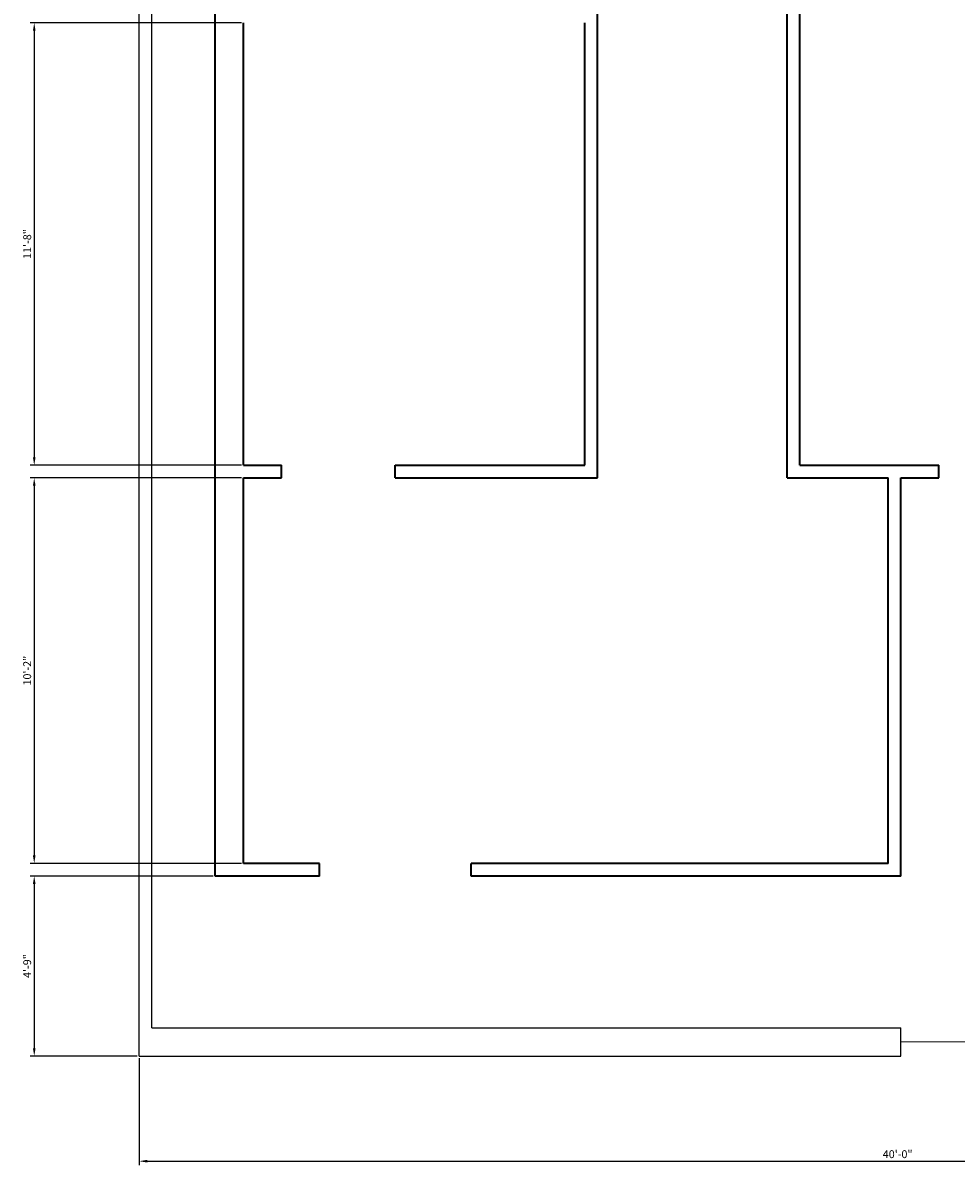
# Model space of a CAD drawing. Units: inches. Extents: x 2169 to 10664, y 1669 to 6352.
# Tile 9 of 17: x 4397 to 4692, y 1968 to 2329. Entities that reach past the tile are written whole.
import ezdxf

# ---------------------------------------------------------------- set-up
doc = ezdxf.new("R2010")
doc.units = ezdxf.units.IN
for name, color, linetype, lineweight in [('A-ANNO-DIMS', 3, 'Continuous', 18), ('A-DOOR', 4, 'Continuous', 18), ('A-WALL', 7, 'Continuous', 35), ('C-PROP', 251, 'Continuous', 25)]:
    doc.layers.add(name, color=color, linetype=linetype, lineweight=lineweight)
doc.styles.get("Standard").update_dxf_attribs({"font": 'arial.ttf'})
doc.dimstyles.new('ISO-25', dxfattribs={"dimtxt": 2.5, "dimasz": 2.5, "dimexe": 1.25, "dimexo": 0.625, "dimtad": 1, "dimdec": 0, "dimlunit": 3, "dimtxsty": 'Standard', "dimcen": 2.5, "dimadec": 0, "dimazin": 0, "dimtfac": 1, "dimtdec": 0, "dimtmove": 0, "dimatfit": 3, "dimfxl": 1, "dimarcsym": 0})

# ---------------------------------------------------------------- blocks, each defined once
blk = doc.blocks.new('*D102')
at = {"layer": 'A-ANNO-DIMS', "color": 0, "lineweight": -2, "transparency": 16777216}
for p, q in [((4433.57, 2001.56), (4433.57, 1967.69)), ((4913.57, 2001.56), (4913.57, 1967.69)), ((4436.07, 1968.94), (4911.07, 1968.94))]:
    blk.add_line(p, q, dxfattribs=at)
at = {"layer": 'A-ANNO-DIMS', "color": 0, "transparency": 16777216}
for points in [[(4436.07, 1969.36), (4436.07, 1968.52), (4433.57, 1968.94)], [(4911.07, 1969.36), (4911.07, 1968.52), (4913.57, 1968.94)]]:
    blk.add_solid(points, dxfattribs=at)
at = {"layer": 'Defpoints', "color": 0, "transparency": 16777216}
for p in [(4433.57, 2002.19), (4913.57, 2002.19), (4913.57, 1968.94)]:
    blk.add_point(p, dxfattribs=at)
at = {"layer": 'A-ANNO-DIMS', "color": 0, "transparency": 16777216, "insert": (4673.57, 1970.84), "char_height": 2.5, "attachment_point": 5}
blk.add_mtext('40\'-0"', dxfattribs=at)
blk = doc.blocks.new('*D114')
at = {"layer": 'A-ANNO-DIMS', "color": 0, "lineweight": -2, "transparency": 16777216}
for p, q in [((4465.95, 2329.19), (4399.07, 2329.19)), ((4400.32, 2326.69), (4400.32, 2191.69)), ((4465.95, 2189.19), (4399.07, 2189.19))]:
    blk.add_line(p, q, dxfattribs=at)
at = {"layer": 'A-ANNO-DIMS', "color": 0, "transparency": 16777216}
for points in [[(4399.91, 2326.69), (4400.74, 2326.69), (4400.32, 2329.19)], [(4399.91, 2191.69), (4400.74, 2191.69), (4400.32, 2189.19)]]:
    blk.add_solid(points, dxfattribs=at)
at = {"layer": 'Defpoints', "color": 0, "transparency": 16777216}
for p in [(4466.57, 2329.19), (4400.32, 2189.19), (4466.57, 2189.19)]:
    blk.add_point(p, dxfattribs=at)
at = {"layer": 'A-ANNO-DIMS', "color": 0, "transparency": 16777216, "insert": (4398.42, 2259.19), "char_height": 2.5, "attachment_point": 5, "rotation": 90}
blk.add_mtext('11\'-8"', dxfattribs=at)
blk = doc.blocks.new('*D115')
at = {"layer": 'A-ANNO-DIMS', "color": 0, "lineweight": -2, "transparency": 16777216}
for p, q in [((4465.95, 2185.19), (4399.07, 2185.19)), ((4400.32, 2182.69), (4400.32, 2065.69)), ((4465.95, 2063.19), (4399.07, 2063.19))]:
    blk.add_line(p, q, dxfattribs=at)
at = {"layer": 'A-ANNO-DIMS', "color": 0, "transparency": 16777216}
for points in [[(4399.91, 2182.69), (4400.74, 2182.69), (4400.32, 2185.19)], [(4399.91, 2065.69), (4400.74, 2065.69), (4400.32, 2063.19)]]:
    blk.add_solid(points, dxfattribs=at)
at = {"layer": 'Defpoints', "color": 0, "transparency": 16777216}
for p in [(4466.57, 2185.19), (4400.32, 2063.19), (4466.57, 2063.19)]:
    blk.add_point(p, dxfattribs=at)
at = {"layer": 'A-ANNO-DIMS', "color": 0, "transparency": 16777216, "insert": (4398.42, 2124.19), "char_height": 2.5, "attachment_point": 5, "rotation": 90}
blk.add_mtext('10\'-2"', dxfattribs=at)
blk = doc.blocks.new('*D116')
at = {"layer": 'A-ANNO-DIMS', "color": 0, "lineweight": -2, "transparency": 16777216}
for p, q in [((4456.95, 2059.19), (4399.07, 2059.19)), ((4400.32, 2056.69), (4400.32, 2004.69)), ((4432.95, 2002.19), (4399.07, 2002.19))]:
    blk.add_line(p, q, dxfattribs=at)
at = {"layer": 'A-ANNO-DIMS', "color": 0, "transparency": 16777216}
for points in [[(4399.91, 2056.69), (4400.74, 2056.69), (4400.32, 2059.19)], [(4399.91, 2004.69), (4400.74, 2004.69), (4400.32, 2002.19)]]:
    blk.add_solid(points, dxfattribs=at)
at = {"layer": 'Defpoints', "color": 0, "transparency": 16777216}
for p in [(4457.57, 2059.19), (4400.32, 2002.19), (4433.57, 2002.19)]:
    blk.add_point(p, dxfattribs=at)
at = {"layer": 'A-ANNO-DIMS', "color": 0, "transparency": 16777216, "insert": (4398.42, 2030.69), "char_height": 2.5, "attachment_point": 5, "rotation": 90}
blk.add_mtext('4\'-9"', dxfattribs=at)

msp = doc.modelspace()

# ---------------------------------------------------------------- linework, layer by layer
at = {"layer": 'A-DOOR'}
msp.add_line((4674.57, 2006.69), (4746.57, 2006.69), dxfattribs=at)
at = {"layer": 'A-WALL'}
for p, q in [((4457.57, 2059.19), (4457.57, 2596.19)), ((4638.57, 2185.19), (4638.57, 2405.19)), ((4642.57, 2189.19), (4642.57, 2405.19)), ((4578.57, 2185.19), (4578.57, 2333.19)), ((4466.57, 2189.19), (4466.57, 2329.19)), ((4574.57, 2189.19), (4574.57, 2329.19)), ((4466.57, 2189.19), (4478.57, 2189.19)), ((4478.57, 2185.19), (4478.57, 2189.19)), ((4514.57, 2185.19), (4514.57, 2189.19)), ((4514.57, 2189.19), (4574.57, 2189.19)), ((4642.57, 2189.19), (4686.57, 2189.19)), ((4686.57, 2185.19), (4686.57, 2189.19)), ((4466.57, 2063.19), (4466.57, 2185.19)), ((4466.57, 2185.19), (4478.57, 2185.19)), ((4514.57, 2185.19), (4578.57, 2185.19)), ((4638.57, 2185.19), (4670.57, 2185.19)), ((4670.57, 2063.19), (4670.57, 2185.19)), ((4674.57, 2059.19), (4674.57, 2185.19)), ((4674.57, 2185.19), (4686.57, 2185.19)), ((4490.57, 2063.19), (4466.57, 2063.19)), ((4490.57, 2059.19), (4490.57, 2063.19)), ((4670.57, 2063.19), (4538.57, 2063.19)), ((4538.57, 2059.19), (4538.57, 2063.19)), ((4490.57, 2059.19), (4457.57, 2059.19)), ((4674.57, 2059.19), (4538.57, 2059.19))]:
    msp.add_line(p, q, dxfattribs=at)
at = {"layer": 'C-PROP'}
for p, q in [((4433.57, 2002.19), (4433.57, 2620.19)), ((4437.57, 2011.19), (4437.57, 2616.19)), ((4437.57, 2011.19), (4674.57, 2011.19)), ((4674.57, 2002.19), (4674.57, 2011.19)), ((4433.57, 2002.19), (4674.57, 2002.19))]:
    msp.add_line(p, q, dxfattribs=at)

# ---------------------------------------------------------------- dimensions: what is measured, and where the dimension line sits
at = {"layer": 'A-ANNO-DIMS'}
for base, p1, p2, picture, middle in [((4400.32, 2189.19), (4466.57, 2329.19), (4466.57, 2189.19), '*D114', (4398.42, 2259.19)), ((4400.32, 2063.19), (4466.57, 2185.19), (4466.57, 2063.19), '*D115', (4398.42, 2124.19)), ((4400.32, 2002.19), (4457.57, 2059.19), (4433.57, 2002.19), '*D116', (4398.42, 2030.69))]:
    dim = msp.add_linear_dim(base=base, p1=p1, p2=p2, angle=90, dimstyle='ISO-25', override={"dimdec": 1, "dimlfac": 1, "dimrnd": 0, "dimzin": 1, "dimdsep": 46, "dimlunit": 4, "dimfrac": 2}, dxfattribs=at)
    dim.commit()
    dim.dimension.update_dxf_attribs({"geometry": picture, "text_midpoint": middle})
dim = msp.add_linear_dim(base=(4913.57, 1968.94), p1=(4433.57, 2002.19), p2=(4913.57, 2002.19), dimstyle='ISO-25', override={"dimdec": 1, "dimlfac": 1, "dimrnd": 0, "dimzin": 1, "dimdsep": 46, "dimlunit": 4, "dimfrac": 2}, dxfattribs=at)
dim.commit()
dim.dimension.update_dxf_attribs({"geometry": '*D102', "text_midpoint": (4673.57, 1970.84)})

doc.saveas('drawing.dxf')
